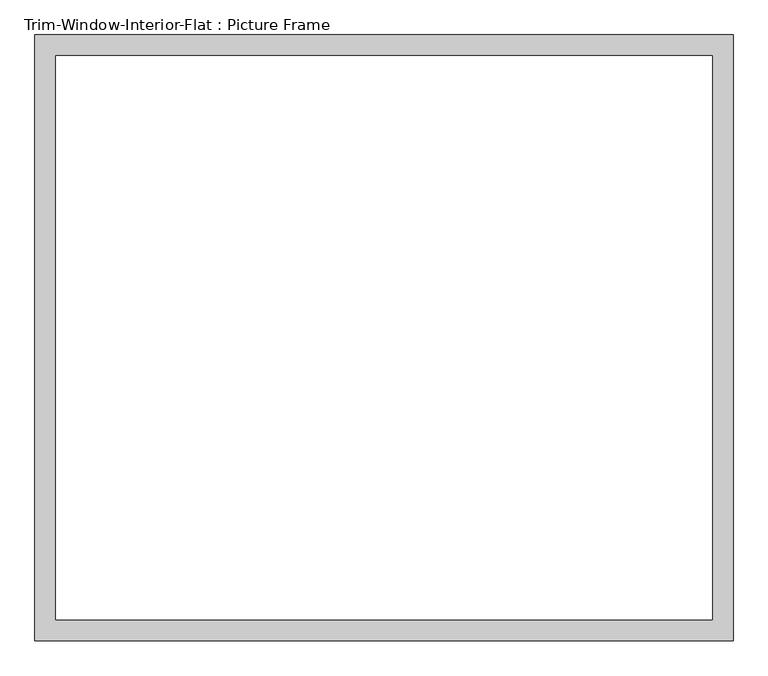
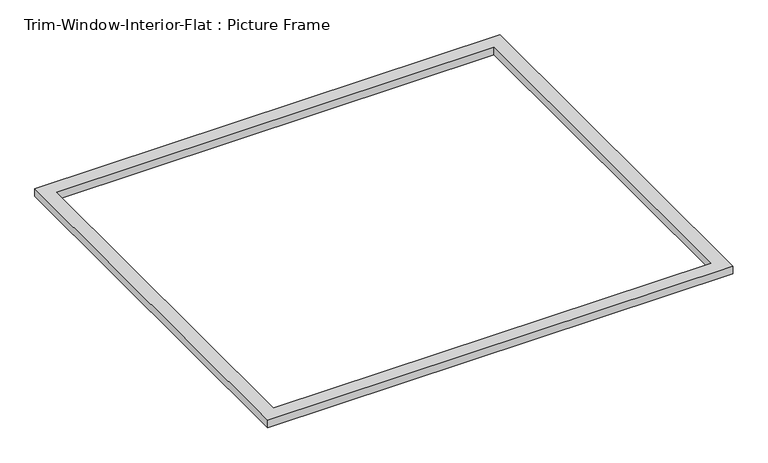
"""IFC4 building model written with IfcOpenShell, lengths in millimetres: proxy geometry, Trim-Window-Interior-Flat : Picture Frame."""

from ifc_helpers import new_model, si_unit, origin, origin_with_axes, place, context, project, spatial, polyline, outline, extrude, source, transform, mapped, element, save


def trim_window_interior_flat_picture_frame_bf12a1e4(model_context):
    return source(origin(), model_context, "Body", "SweptSolid", [
        extrude(outline(polyline([(958.85, 44.45), (958.85, -1619.25), (-958.85, -1619.25), (-958.85, 44.45), (958.85, 44.45)]), holes=[polyline([(901.7, -12.7), (-901.7, -12.7), (-901.7, -1562.1), (901.7, -1562.1), (901.7, -12.7)])]), origin_with_axes(), (0.0, 0.0, 1.0), 31.75),
    ])


if __name__ == "__main__":
    model = new_model("IFC4")
    model_context = context("Model", 3, world=origin())
    ifc_project = project(units=[si_unit("LENGTHUNIT", "METRE", prefix="MILLI")], contexts=[model_context])
    site = spatial("IfcSite", under=ifc_project)
    building = spatial("IfcBuilding", under=site)
    placement = place(None, origin())
    trim_window_interior_flat_picture_frame_shape = trim_window_interior_flat_picture_frame_bf12a1e4(model_context)
    element("IfcBuildingElementProxy", 1, Name="Trim-Window-Interior-Flat : Picture Frame", ObjectType="Trim-Window-Interior-Flat : Picture Frame", at=placement, inside=building, context=model_context, shape_type="MappedRepresentation", body=[
        mapped(trim_window_interior_flat_picture_frame_shape, transform((0.0, 0.0, 0.0), x_axis=(1.0, 0.0, 0.0), y_axis=(0.0, 1.0, 0.0), z_axis=(0.0, 0.0, 1.0))),
    ])
    save(model, "model.ifc")

# Revit data of these elements
# Type "Trim-Window-Interior-Flat : Picture Frame"
#   Trim Thickness_Picture Frame = 0' - 1 1/4"
#   Trim Width = 0' - 2 1/4"
#   Trim Thickness_with Sill = 0' - 0 3/4"
#   Sill Thickness = 0' - 1 1/4"
#   Opening Width [instance default] = 2' - 0"
#   Opening Height [instance default] = 3' - 0"
#   Default Elevation = 4' - 0"
#   Sill = no
#   Picture Frame = yes
#   Trim Material [instance default] = none
# Element 1 (IfcBuildingElementProxy, "Trim-Window-Interior-Flat : Picture Frame")
#   Opening Width = 6' - 0"
#   Opening Height = 5' - 2"
#   Trim Material = Wood - Stained
#   Materials on its faces: "Wood - Stained"
# Materials
#   "Wood - Stained": class "Wood", colour RGB 224 178 126, transparency 0, Cost = 0
